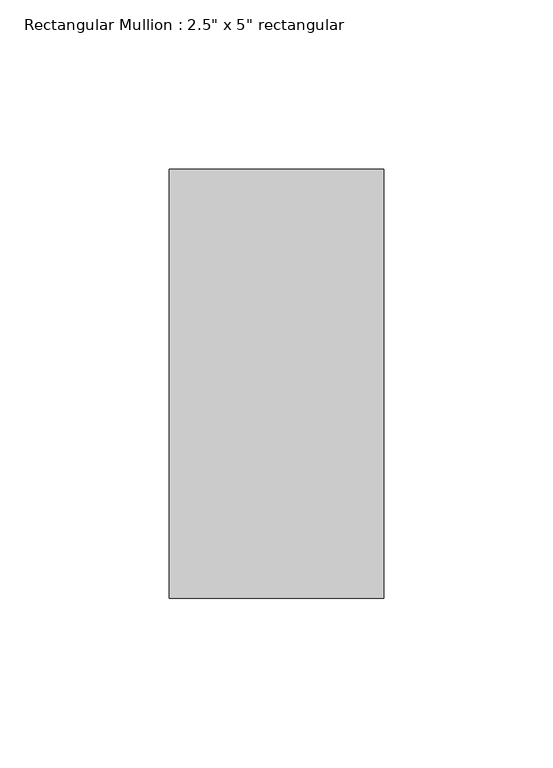
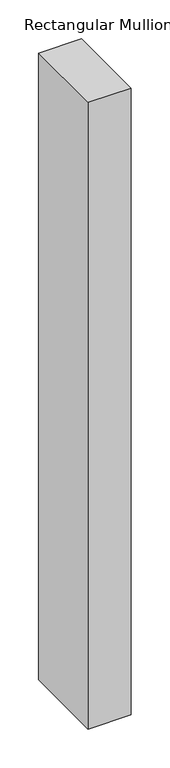
"""IFC4 building model written with IfcOpenShell, lengths in millimetres: member geometry."""

from ifc_helpers import new_model, si_unit, frame, origin, place, context, project, spatial, polyline, outline, extrude, source, transform, mapped, element, save


def member_8d384f73(model_context):
    return source(origin(), model_context, "Body", "SweptSolid", [
        extrude(outline(polyline([(0.0, 63.5), (0.0, -63.5), (-63.5, -63.5), (-63.5, 63.5), (0.0, 63.5)])), frame((0.0, 0.0, -983.0744987), z_axis=(0.0, 0.0, 1.0), x_axis=(1.0, 0.0, 0.0)), (0.0, 0.0, 1.0), 983.0744987),
    ])


if __name__ == "__main__":
    model = new_model("IFC4")
    model_context = context("Model", 3, world=origin())
    ifc_project = project(units=[si_unit("LENGTHUNIT", "METRE", prefix="MILLI")], contexts=[model_context])
    site = spatial("IfcSite", under=ifc_project)
    building = spatial("IfcBuilding", under=site)
    placement = place(None, origin())
    member_shape = member_8d384f73(model_context)
    element("IfcMember", 1, ObjectType="Rectangular Mullion : 2.5\" x 5\" rectangular", at=placement, inside=building, context=model_context, shape_type="MappedRepresentation", body=[
        mapped(member_shape, transform((0.0, 0.0, 0.0), x_axis=(1.0, 0.0, 0.0), y_axis=(0.0, 1.0, 0.0), z_axis=(0.0, 0.0, 1.0))),
    ])
    save(model, "model.ifc")

# Revit data of these elements
# Type "Rectangular Mullion : 2.5\" x 5\" rectangular"
#   built-in parameter 1007304 = 0.416667 (stored number, unit not read)
#   built-in parameter 1007301 = 0.104167 (stored number, unit not read)
#   built-in parameter 1007300 = 0.104167 (stored number, unit not read)
# Element 1 (IfcMember, "Rectangular Mullion : 2.5\" x 5\" rectangular")
#   Materials on its faces: "Aluminum"
# Materials
#   "Aluminum": class "Metal", colour RGB 247 247 247, transparency 0, Description = "Aluminum 6061", Cost = 0
